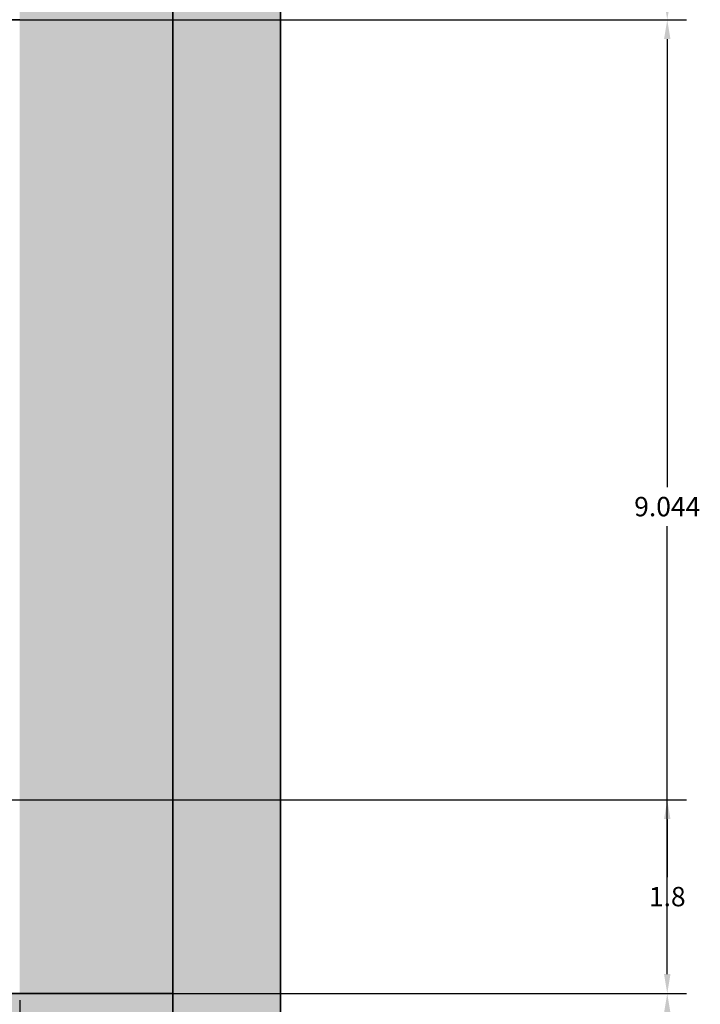
# Model space of a CAD drawing. Units: inches. Extents: x 18 to 59.8, y 2.7 to 81.2.
# Tile 6 of 9: x 53.4 to 59.8, y 29.5 to 38.7. Entities that reach past the tile are written whole.
import ezdxf

# ---------------------------------------------------------------- set-up
doc = ezdxf.new("R2010")
doc.units = ezdxf.units.IN
doc.header["$MEASUREMENT"] = 0
for name, color, linetype, lineweight in [('A-ANNO-DIMS', 2, 'Continuous', 18), ('A-ELEV', 7, 'Continuous', 35), ('A-ELEV-PATT', 8, 'Continuous', 13)]:
    doc.layers.add(name, color=color, linetype=linetype, lineweight=lineweight)
doc.styles.get("Standard").update_dxf_attribs({"font": 'arial.ttf'})
doc.dimstyles.get("Standard").update_dxf_attribs({"dimtxt": 0.18, "dimasz": 0.18, "dimexe": 0.18, "dimexo": 0.0625, "dimgap": 0.09, "dimtad": 0, "dimtih": 1, "dimtoh": 1, "dimdec": 1, "dimzin": 0, "dimdsep": 46, "dimlunit": 3, "dimtxsty": 'Standard', "dimcen": 0.09, "dimadec": 0, "dimazin": 0, "dimtfac": 1, "dimtdec": 1, "dimtofl": 0, "dimtmove": 0, "dimatfit": 3, "dimfxl": 1, "dimtolj": 1, "dimtzin": 0, "dimarcsym": 0})

# ---------------------------------------------------------------- blocks, each defined once
blk = doc.blocks.new('*D15')
at = {"layer": 'A-ANNO-DIMS', "color": 0, "lineweight": -2, "transparency": 16777216}
for p, q in [((54.92247100000003, 29.64074800000001), (59.62997100000006, 29.64074800000002)), ((59.44997100000005, 29.46074800000002), (59.44997100000005, 26.12074800000002)), ((59.44997100000005, 22.42074800000001), (59.44997100000005, 25.76074800000001)), ((55.92247100000003, 22.24074800000001), (59.62997100000006, 22.24074800000001))]:
    blk.add_line(p, q, dxfattribs=at)
at = {"layer": 'A-ANNO-DIMS', "color": 0, "transparency": 16777216}
for points in [[(59.41997100000005, 29.46074800000002), (59.47997100000005, 29.46074800000002), (59.44997100000005, 29.64074800000002)], [(59.41997100000005, 22.42074800000001), (59.47997100000005, 22.42074800000001), (59.44997100000005, 22.24074800000001)]]:
    blk.add_solid(points, dxfattribs=at)
at = {"layer": 'Defpoints', "color": 0, "transparency": 16777216}
for p in [(54.85997100000003, 29.64074800000001), (59.44997100000005, 29.64074800000002), (55.85997100000003, 22.24074800000001)]:
    blk.add_point(p, dxfattribs=at)
at = {"layer": 'A-ANNO-DIMS', "color": 0, "transparency": 16777216, "insert": (59.44997100000005, 25.94074799999999), "char_height": 0.18, "attachment_point": 5}
blk.add_mtext('\\A1;7.4', dxfattribs=at)
blk = doc.blocks.new('*D16')
at = {"layer": 'A-ANNO-DIMS', "color": 0, "lineweight": -2, "transparency": 16777216}
for p, q in [((53.50256100000002, 38.68456300000001), (59.62997100000006, 38.68456300000001)), ((59.44997100000005, 38.50456300000001), (59.44997100000005, 34.34455863778992)), ((59.44997100000005, 29.82074800000002), (59.44997100000005, 33.98075236221011)), ((54.92247100000003, 29.64074800000001), (59.62997100000006, 29.64074800000002))]:
    blk.add_line(p, q, dxfattribs=at)
at = {"layer": 'A-ANNO-DIMS', "color": 0, "transparency": 16777216}
for points in [[(59.41997100000005, 38.50456300000001), (59.47997100000005, 38.50456300000001), (59.44997100000005, 38.68456300000001)], [(59.41997100000005, 29.82074800000002), (59.47997100000005, 29.82074800000002), (59.44997100000005, 29.64074800000002)]]:
    blk.add_solid(points, dxfattribs=at)
at = {"layer": 'Defpoints', "color": 0, "transparency": 16777216}
for p in [(53.44006100000003, 38.68456300000001), (59.44997100000005, 38.68456300000001), (54.85997100000003, 29.64074800000001)]:
    blk.add_point(p, dxfattribs=at)
at = {"layer": 'A-ANNO-DIMS', "color": 0, "transparency": 16777216, "insert": (59.44997100000005, 34.16265549999998), "char_height": 0.18, "attachment_point": 5}
blk.add_mtext('\\A1;9.044', dxfattribs=at)
blk = doc.blocks.new('*D17')
at = {"layer": 'A-ANNO-DIMS', "color": 0, "lineweight": -2, "transparency": 16777216}
for p, q in [((53.50256100000002, 48.44074800000003), (59.62997100000005, 48.44074800000003)), ((59.44997100000005, 48.26074800000003), (59.44997100000005, 43.74455863778991)), ((59.44997100000005, 38.86456300000001), (59.44997100000005, 43.38075236221011)), ((53.50256100000002, 38.68456300000001), (59.62997100000006, 38.68456300000001))]:
    blk.add_line(p, q, dxfattribs=at)
at = {"layer": 'A-ANNO-DIMS', "color": 0, "transparency": 16777216}
for points in [[(59.41997100000005, 48.26074800000003), (59.47997100000005, 48.26074800000003), (59.44997100000005, 48.44074800000003)], [(59.41997100000005, 38.86456300000001), (59.47997100000005, 38.86456300000001), (59.44997100000005, 38.68456300000001)]]:
    blk.add_solid(points, dxfattribs=at)
at = {"layer": 'Defpoints', "color": 0, "transparency": 16777216}
for p in [(53.44006100000003, 48.44074800000003), (59.44997100000005, 48.44074800000003), (53.44006100000003, 38.68456300000001)]:
    blk.add_point(p, dxfattribs=at)
at = {"layer": 'A-ANNO-DIMS', "color": 0, "transparency": 16777216, "insert": (59.44997100000005, 43.56265549999998), "char_height": 0.18, "attachment_point": 5}
blk.add_mtext('\\A1;9.756', dxfattribs=at)
blk = doc.blocks.new('*D23')
at = {"layer": 'A-ANNO-DIMS', "color": 0, "lineweight": -2, "transparency": 16777216}
for p, q in [((48.859971, 29.578248), (48.859971, 2.670747999999999)), ((53.440061, 29.578248), (53.440061, 2.670747999999999)), ((49.039971, 2.850747999999999), (50.82243073396998, 2.850747999999999)), ((53.260061, 2.850747999999999), (51.47760126603001, 2.850747999999999))]:
    blk.add_line(p, q, dxfattribs=at)
at = {"layer": 'A-ANNO-DIMS', "color": 0, "transparency": 16777216}
for points in [[(49.039971, 2.880747999999999), (49.039971, 2.820748), (48.859971, 2.850747999999999)], [(53.260061, 2.880747999999999), (53.260061, 2.820748), (53.440061, 2.850747999999999)]]:
    blk.add_solid(points, dxfattribs=at)
at = {"layer": 'Defpoints', "color": 0, "transparency": 16777216}
for p in [(48.859971, 29.640748), (53.440061, 29.640748), (53.440061, 2.850747999999999)]:
    blk.add_point(p, dxfattribs=at)
at = {"layer": 'A-ANNO-DIMS', "color": 0, "transparency": 16777216, "insert": (51.150016, 2.850747999999999), "char_height": 0.18, "attachment_point": 5}
blk.add_mtext('\\A1;4.58', dxfattribs=at)
blk = doc.blocks.new('*D26')
at = {"layer": 'A-ANNO-DIMS', "color": 0, "lineweight": -2, "transparency": 16777216}
for p, q in [((52.98946600000003, 41.31595800000002), (59.62997100000006, 41.31595800000002)), ((59.44997100000005, 41.13595800000001), (59.44997100000005, 40.18222502933153)), ((59.44997100000005, 38.86456300000001), (59.44997100000005, 39.8182959706685)), ((52.98946600000003, 38.68456300000001), (59.62997100000006, 38.68456300000001))]:
    blk.add_line(p, q, dxfattribs=at)
at = {"layer": 'A-ANNO-DIMS', "color": 0, "transparency": 16777216}
for points in [[(59.41997100000005, 41.13595800000001), (59.47997100000005, 41.13595800000001), (59.44997100000005, 41.31595800000002)], [(59.41997100000005, 38.86456300000001), (59.47997100000005, 38.86456300000001), (59.44997100000005, 38.68456300000001)]]:
    blk.add_solid(points, dxfattribs=at)
at = {"layer": 'Defpoints', "color": 0, "transparency": 16777216}
for p in [(52.92696600000002, 41.31595800000002), (59.44997100000005, 41.31595800000002), (52.92696600000002, 38.68456300000001)]:
    blk.add_point(p, dxfattribs=at)
at = {"layer": 'A-ANNO-DIMS', "color": 0, "transparency": 16777216, "insert": (59.44997100000005, 40.00026049999998), "char_height": 0.18, "attachment_point": 5}
blk.add_mtext('\\A1;2.63', dxfattribs=at)
blk = doc.blocks.new('*D27')
at = {"layer": 'A-ANNO-DIMS', "color": 0, "lineweight": -2, "transparency": 16777216}
for p, q in [((30.46859000000001, 31.44074800000002), (59.62997100000006, 31.44074800000002)), ((59.44997100000005, 31.26074800000002), (59.44997100000005, 30.72265113778992)), ((59.44997100000005, 29.82074800000002), (59.44997100000005, 30.35884486221011)), ((48.92247100000003, 29.64074800000001), (59.62997100000006, 29.64074800000002))]:
    blk.add_line(p, q, dxfattribs=at)
at = {"layer": 'A-ANNO-DIMS', "color": 0, "transparency": 16777216}
for points in [[(59.41997100000005, 31.26074800000002), (59.47997100000005, 31.26074800000002), (59.44997100000005, 31.44074800000002)], [(59.41997100000005, 29.82074800000002), (59.47997100000005, 29.82074800000002), (59.44997100000005, 29.64074800000002)]]:
    blk.add_solid(points, dxfattribs=at)
at = {"layer": 'Defpoints', "color": 0, "transparency": 16777216}
for p in [(30.40609000000002, 31.44074800000002), (48.85997100000003, 29.64074800000001), (59.44997100000005, 29.64074800000002)]:
    blk.add_point(p, dxfattribs=at)
at = {"layer": 'A-ANNO-DIMS', "color": 0, "transparency": 16777216, "insert": (59.44997100000005, 30.54074799999999), "char_height": 0.18, "attachment_point": 5}
blk.add_mtext('\\A1;1.8', dxfattribs=at)

msp = doc.modelspace()

# ---------------------------------------------------------------- hatches: boundary and pattern name
at = {"layer": 'A-ELEV-PATT'}
h = msp.add_hatch(color=256, dxfattribs=at)
h.set_gradient(color1=(255, 255, 255), color2=(199, 200, 202))
h.paths.add_polyline_path([(38.85997087182833, 75.45212783007513, 0.4125526599533602), (36.85997087192615, 77.44074750583997), (21.85997087182832, 77.44074750583995), (21.85997087182832, 22.44074750583995), (22.85997087182833, 22.44074750583995), (48.85997087182833, 22.44074750583996), (48.85997087182833, 30.92342676155402, 0.4074472928332927), (48.33023903111634, 31.44074750583995), (30.40609029701442, 31.44074750583996, -0.7603989452129261), (34.01164157247843, 44.44074750583996), (47.85997087182832, 44.44074750583995, -0.4142135623730951), (48.85997087182833, 43.44074750583994), (48.85997087182833, 48.44074750583995, 0.4142135623730955), (47.85997087182832, 49.44074750583995), (32.23382408177119, 49.44074750583993, -0.2243141867862321), (27.84111392101349, 52.84266085519661, -0.8480128940945467), (38.85997087182833, 61.44074750583993)])
h.paths.add_polyline_path([(55.85997087182832, 77.44074750583995), (54.85997087182832, 77.44074750583997), (54.85997087182832, 22.24074750583996), (55.85997087182832, 22.24074750583995)])
h.paths.add_polyline_path([(54.85997087182832, 51.54074750583995), (53.44006084017791, 51.54074750583996), (53.44006084017792, 29.64074750583996), (54.85997087182832, 29.64074750583996)])
h.paths.add_polyline_path([(54.85997087182832, 61.44074750583993), (53.44006084017791, 57.44074750583993), (53.44006084017791, 51.64074750583996), (54.85997087182832, 51.64074750583996)])
h.paths.add_polyline_path([(54.85997087182832, 29.44074750583995), (54.47100875861361, 29.44074750583995), (54.47100875861361, 22.24074750583996), (54.85997087182832, 22.24074750583996)])
h.paths.add_polyline_path([(55.57447446325177, 22.24074750583995), (54.85997087182832, 22.24074750583996), (54.57447446325178, 22.24074750583996), (53.93466996146642, 21.792542566958), (54.58769880335594, 21.54947740208223)])
h.paths.add_polyline_path([(54.59913950424823, 21.54521903603421), (53.94430429933965, 21.78895655088426), (53.94430429933965, 18.44074750583995), (54.59913950424823, 18.44074750583995)])
h.paths.add_polyline_path([(53.94430429933965, 21.78895655088427), (53.93466996146642, 21.792542566958), (53.58162006229036, 21.54521903603422), (53.58162006229036, 18.44074750583995), (53.94430429933965, 18.44074750583994)])
h.paths.add_polyline_path([(53.36475139777029, 20.69276091189374), (52.89555240690669, 21.06460517556268), (52.89555240690669, 18.44074750583995), (53.3647513977703, 18.44074750583994)])
h.paths.add_polyline_path([(52.89555240690669, 21.06460517556268), (50.57752474318004, 19.44074750583995), (50.57752474318004, 18.44074750583995), (52.89555240690669, 18.44074750583995)])
h.paths.add_polyline_path([(53.58162006229036, 21.54521903603423), (52.89555240690668, 21.06460517556268), (53.3647513977703, 20.69276091189373), (53.58162006229036, 20.84468482967704)])
h.paths.add_polyline_path([(26.81093959479239, 19.44074750583995), (24.96715419074249, 20.84074750583995), (24.96715419074249, 18.44074750583995), (26.81093959479239, 18.44074750583995)])
h.paths.add_polyline_path([(24.96715419074249, 20.84074750583995), (24.41645576890079, 20.84268308307895), (24.41645576890079, 18.44074750583994), (24.96715419074249, 18.44074750583994)])
h.paths.add_polyline_path([(24.41645576890079, 20.84268308307895), (24.41645576890079, 21.25889692219009), (24.05877847081848, 21.5304839605815), (24.03006070560372, 21.51834150822755), (24.03006070560372, 18.44074750583995), (24.41645576890079, 18.44074750583995)])
h.paths.add_polyline_path([(24.03006070560372, 21.51834150822755), (23.41645576890078, 21.2588969221901), (23.41645576890078, 18.44074750583996), (24.03006070560372, 18.44074750583995)])
h.paths.add_polyline_path([(24.03006070560372, 21.51834150822755), (24.05877847081849, 21.53048396058151), (23.12336878669258, 22.24074750583995), (22.12336878669259, 22.24074750583996), (23.41645576890079, 21.2588969221901)])
h.paths.add_polyline_path([(24.41645576890079, 21.2588969221901), (24.41645576890079, 20.84268308307896), (24.96715419074249, 20.84074750583994)])
h.paths.add_polyline_path([(47.85997087182832, 18.44074750583995), (29.85997087182832, 18.44074750583995), (29.85997087182832, 6.440747505839951), (30.85997087182832, 6.440747505839937), (30.85997087182832, 17.44074750583995), (38.85997087182833, 17.44074750583995), (46.85997087182832, 17.44074750583995), (46.85997087182832, 6.440747505839937), (47.85997087182832, 6.440747505839958)])
h.paths.add_polyline_path([(54.57559250001032, 15.2149800477124), (54.57559250001032, 6.440747505839944), (55.85997087182832, 6.440747505839951), (55.85997087182832, 18.44074750583995), (47.85997087182832, 18.44074750583995), (47.85997087182832, 6.440747505839944), (49.14824210254597, 6.440747505839944), (49.14824210254597, 15.2149800477124, -1)])
h = msp.add_hatch(color=256, dxfattribs=at)
h.paths.add_polyline_path([(27.84111392101356, 52.84266085519647, -0.7443789445921651), (36.85997087182832, 61.44074750583993), (38.85997087182833, 61.44074750583993, 0.8480128940945556)])
h.paths.add_polyline_path([(47.85997087182832, 44.44074750583995), (34.01164157247843, 44.44074750583996, 0.7603989452129407), (30.40609029701462, 31.44074750583983, -0.7376245609052545), (34.01164157247731, 43.44074750583994), (47.85997087182831, 43.44074750583994, -0.4142135623730951), (48.85997087182832, 42.44074750583995), (48.85997087182833, 43.44074750583994, 0.4142135623730951)])
h.paths.add_polyline_path([(54.57559250001032, 15.2149800477124), (54.57559250001032, 6.440747505839951), (55.85997087182832, 6.440747505839951), (55.85997087182832, 18.44074750583995), (47.85997087182832, 18.44074750583995), (47.85997087182832, 6.440747505839944), (49.14824210254597, 6.440747505839944), (49.14824210254597, 15.2149800477124, -1)])
h.paths.add_polyline_path([(47.85997087182832, 18.44074750583995), (29.85997087182832, 18.44074750583995), (29.85997087182832, 6.440747505839958), (30.85997087182832, 6.440747505839951), (30.85997087182832, 17.44074750583995), (38.85997087182833, 17.44074750583995), (46.85997087182832, 17.44074750583995), (46.85997087182832, 6.440747505839944), (47.85997087182832, 6.440747505839951)])
h.paths.add_polyline_path([(55.85997087182832, 77.44074750583995), (54.85997087182832, 77.44074750583997), (54.85997087182833, 22.24074750583995), (55.85997087182832, 22.24074750583995)])
h = msp.add_hatch(dxfattribs=at)
h.set_pattern_fill('ANSI31', color=256, scale=5, angle=45, style=0)
h.set_pattern_definition([(90, (0, 0), (-0.6250000000000001, 0), [])])
h.paths.add_polyline_path([(54.85997087182832, 69.44074750583995), (38.85997087182833, 69.44074750583995), (38.85997087182833, 61.44074750583995), (54.85997087182832, 61.44074750583994)])
h.paths.add_polyline_path([(54.85997087182833, 61.44074750583994), (38.85997087182833, 61.44074750583995), (36.85997087182832, 61.44074750583993, 0.4434140223301819), (27.69861713021859, 58.44074750583995), (48.85997087182833, 58.44074750583995), (48.85997087182833, 57.44074750583994), (53.44006084017792, 57.44074750583995)])
h.paths.add_polyline_path([(37.16613704638868, 59.85769359025997), (37.11866134610267, 59.85769359025997), (37.11866134610267, 59.93991004599954), (37.49943513222304, 59.93991004599954), (37.49943513222304, 59.85769359025997), (37.45195943193702, 59.85769359025997, -3.476462016968403)], flags=16)
h.paths.add_polyline_path([(42.66000754223224, 59.8390978600294), (42.61253184194623, 59.8390978600294), (42.61253184194623, 59.92131431576897), (42.9933056280666, 59.92131431576897), (42.9933056280666, 59.8390978600294), (42.94582992778058, 59.8390978600294, -3.47646201696846)], flags=16)
h.paths.add_polyline_path([(49.64399186138049, 60.00882068949565), (49.59651616109447, 60.00882068949565), (49.59651616109447, 60.09103714523522), (49.97728994721485, 60.09103714523522), (49.97728994721485, 60.00882068949565), (49.92981424692883, 60.00882068949565, -3.476462016968434)], flags=16)
h.paths.add_polyline_path([(44.46707765301489, 57.04074750583994), (32.6670776530149, 57.04074750583994), (32.6670776530149, 56.04074750583993), (44.46707765301489, 56.04074750583993)])
h.paths.add_polyline_path([(47.85997087182831, 43.44074750583994), (46.85997087182832, 43.44074750583994), (34.0116415724774, 43.44074750583994, 0.2012982920418866), (29.34810857035394, 41.44074750583995), (47.85997087182831, 41.44074750583995, 1)])
h.paths.add_polyline_path([(36.60163289663952, 42.55241488062237), (36.55415719635351, 42.55241488062236), (36.55415719635351, 42.63463133636193), (36.93493098247388, 42.63463133636193), (36.93493098247388, 42.55241488062236), (36.88745528218787, 42.55241488062236, -3.476462016968307)], flags=16)
h.paths.add_polyline_path([(42.98647563665846, 42.5780367704526), (42.93899993637245, 42.5780367704526), (42.93899993637245, 42.66025322619216), (43.31977372249282, 42.66025322619216), (43.31977372249282, 42.57803677045259), (43.2722980222068, 42.57803677045259, -3.476462016968351)], flags=16)
h.paths.add_polyline_path([(54.47100875861361, 29.44074750583995), (48.85997087182833, 29.44074750583995), (48.85997087182833, 22.24074750583995), (54.47100875861361, 22.24074750583994)])
h.paths.add_polyline_path([(54.57447446325179, 22.24074750583995), (23.12336878669258, 22.24074750583995), (26.81093959479238, 19.44074750583996), (50.57752474318005, 19.44074750583996)])
h.paths.add_polyline_path([(54.57559250001032, 15.2149800477124, 1), (49.14824210254597, 15.2149800477124), (49.14824210254597, 6.440747505839958), (54.57559250001032, 6.440747505839944)])
h.paths.add_polyline_path([(49.83226884926398, 9.122455521673542), (49.66565363924473, 9.122455521673537), (49.66565363924473, 12.60204276083839), (49.83226884926398, 12.6020427608384)], flags=16)
h = msp.add_hatch(color=256, dxfattribs=at)
h.paths.add_polyline_path([(38.85997087182833, 17.44074750583995), (30.85997087182832, 17.44074750583995), (30.85997087182832, 6.440747505839954), (30.95997087182833, 6.440747505839954), (30.95997087182833, 17.34074750583995), (38.85997087182833, 17.34074750583995)])
h.paths.add_polyline_path([(46.85997087182832, 17.44074750583995), (38.85997087182833, 17.44074750583995), (38.85997087182833, 17.34074750583995), (46.75997087182832, 17.34074750583994), (46.75997087182832, 6.440747505839953), (46.85997087182832, 6.440747505839953)])
h.paths.add_polyline_path([(49.83226884926398, 12.6020427608384), (49.66565363924473, 12.6020427608384), (49.66565363924473, 9.122455521673542), (49.83226884926398, 9.122455521673542)])
h.paths.add_polyline_path([(48.85997087182833, 22.44074750583996), (21.85997087182832, 22.44074750583995), (21.85997087182832, 22.24074750583995), (48.85997087182833, 22.24074750583995)])
h.paths.add_polyline_path([(54.85997087182833, 29.64074750583995), (48.85997087182833, 29.64074750583995), (48.85997087182833, 29.44074750583995), (54.85997087182832, 29.44074750583995)])
edge = h.paths.add_edge_path()
edge.add_spline(control_points=[(48.33023903111483, 33.5344962306578), (48.12289134557783, 33.67095813700708), (47.91554366004082, 33.80742004335637), (47.68392077892267, 33.83364072465344)], knot_values=[0, 0, 0, 0, 0.7121900809507601, 0.7121900809507601, 0.7121900809507601, 0.7121900809507601], degree=3, periodic=0)
edge.add_line((47.68392077892267, 33.83364072465344), (28.25825772220566, 33.83364072465339))
edge.add_arc((34.06310194306086, 36.88361892210756), 6.557330511217329, 207.718310588115, 208.7099022277735)
edge.add_line((28.31190895474052, 33.73364072465339), (47.62375606275408, 33.73364072465342))
edge.add_spline(control_points=[(47.62375606275404, 33.73364072465342), (47.64610436199382, 33.73406508503794), (47.6684526612336, 33.73448944542246), (47.690500685503, 33.73364072465343)], knot_values=[0, 0, 0, 0, 0.0667446227489563, 0.0667446227489563, 0.0667446227489563, 0.0667446227489563], degree=3, periodic=0)
edge.add_spline(control_points=[(47.690500685503, 33.73364072465343), (47.7384016558997, 33.73179681574185), (47.78488530471712, 33.7239438632234), (47.83023903111267, 33.71130035843739)], knot_values=[0.5701039528936152, 0.5701039528936244, 0.5701039528936244, 0.5701039528936244, 0.7151116034373645, 0.7151116034373645, 0.7151116034373645, 0.7151116034373645], degree=3, periodic=0)
edge.add_spline(control_points=[(47.83023903111267, 33.71130035843739), (48.0085492002631, 33.66159186354143), (48.16939411568897, 33.53783562057542), (48.33023903111483, 33.41407937760941)], knot_values=[0, 0, 0, 0, 0.5701039528936152, 0.5701039528936152, 0.5701039528936152, 0.5701039528936152], degree=3, periodic=0)
edge.add_line((48.33023903111483, 33.41407937760941), (48.33023903111483, 33.5344962306578))

# ---------------------------------------------------------------- linework, layer by layer
at = {"layer": 'A-ELEV'}
for p, q in [((54.85997087182833, 22.24074750583995), (54.85997087182832, 77.44074750583995)), ((55.85997087182832, 77.44074750583994), (55.85997087182832, 22.24074750583995)), ((54.85997087182832, 29.64074750583995), (48.85997087182833, 29.64074750583995))]:
    msp.add_line(p, q, dxfattribs=at)
msp.add_lwpolyline([(53.44006084017792, 38.68456317332766), (48.85997087182833, 38.68456317332766), (48.85997087182833, 29.64074750583995), (54.85997087182832, 29.64074750583995), (54.85997087182832, 38.68456317332766)], dxfattribs=at)

# ---------------------------------------------------------------- dimensions: what is measured, and where the dimension line sits
at = {"layer": 'A-ANNO-DIMS'}
for base, p1, p2, override, picture, middle in [((59.44997100000005, 48.44074800000003), (53.440061, 38.684563), (53.440061, 48.440748), {"dimdec": 3, "dimlfac": 1, "dimrnd": 0, "dimzin": 0, "dimdsep": 46, "dimlunit": 2}, '*D17', (59.44997100000005, 43.56265549999998)), ((59.44997100000005, 41.31595800000002), (52.926966, 38.684563), (52.926966, 41.315958), {"dimdec": 2, "dimlfac": 1, "dimrnd": 0, "dimzin": 0, "dimdsep": 46, "dimlunit": 2}, '*D26', (59.44997100000005, 40.00026049999998)), ((59.44997100000005, 38.68456300000001), (54.859971, 29.640748), (53.440061, 38.684563), {"dimdec": 3, "dimlfac": 1, "dimrnd": 0, "dimzin": 0, "dimdsep": 46, "dimlunit": 2}, '*D16', (59.44997100000005, 34.16265549999998)), ((59.44997100000005, 29.64074800000002), (30.40609, 31.440748), (48.859971, 29.640748), {"dimdec": 1, "dimlfac": 1, "dimrnd": 0, "dimzin": 0, "dimdsep": 46, "dimlunit": 2}, '*D27', (59.44997100000005, 30.54074799999999)), ((59.44997100000005, 29.64074800000002), (55.859971, 22.240748), (54.859971, 29.640748), {"dimdec": 1, "dimlfac": 1, "dimrnd": 0, "dimzin": 0, "dimdsep": 46, "dimlunit": 2}, '*D15', (59.44997100000005, 25.94074799999999))]:
    dim = msp.add_linear_dim(base=base, p1=p1, p2=p2, angle=90, dimstyle='Standard', override=override, dxfattribs=at)
    dim.commit()
    dim.dimension.update_dxf_attribs({"geometry": picture, "text_midpoint": middle})
dim = msp.add_linear_dim(base=(53.440061, 2.850747999999999), p1=(48.859971, 29.640748), p2=(53.440061, 29.640748), dimstyle='Standard', override={"dimdec": 2, "dimlfac": 1, "dimrnd": 0, "dimzin": 0, "dimdsep": 46, "dimlunit": 2}, dxfattribs=at)
dim.commit()
dim.dimension.update_dxf_attribs({"geometry": '*D23', "text_midpoint": (51.150016, 2.850747999999999)})

doc.saveas('drawing.dxf')
